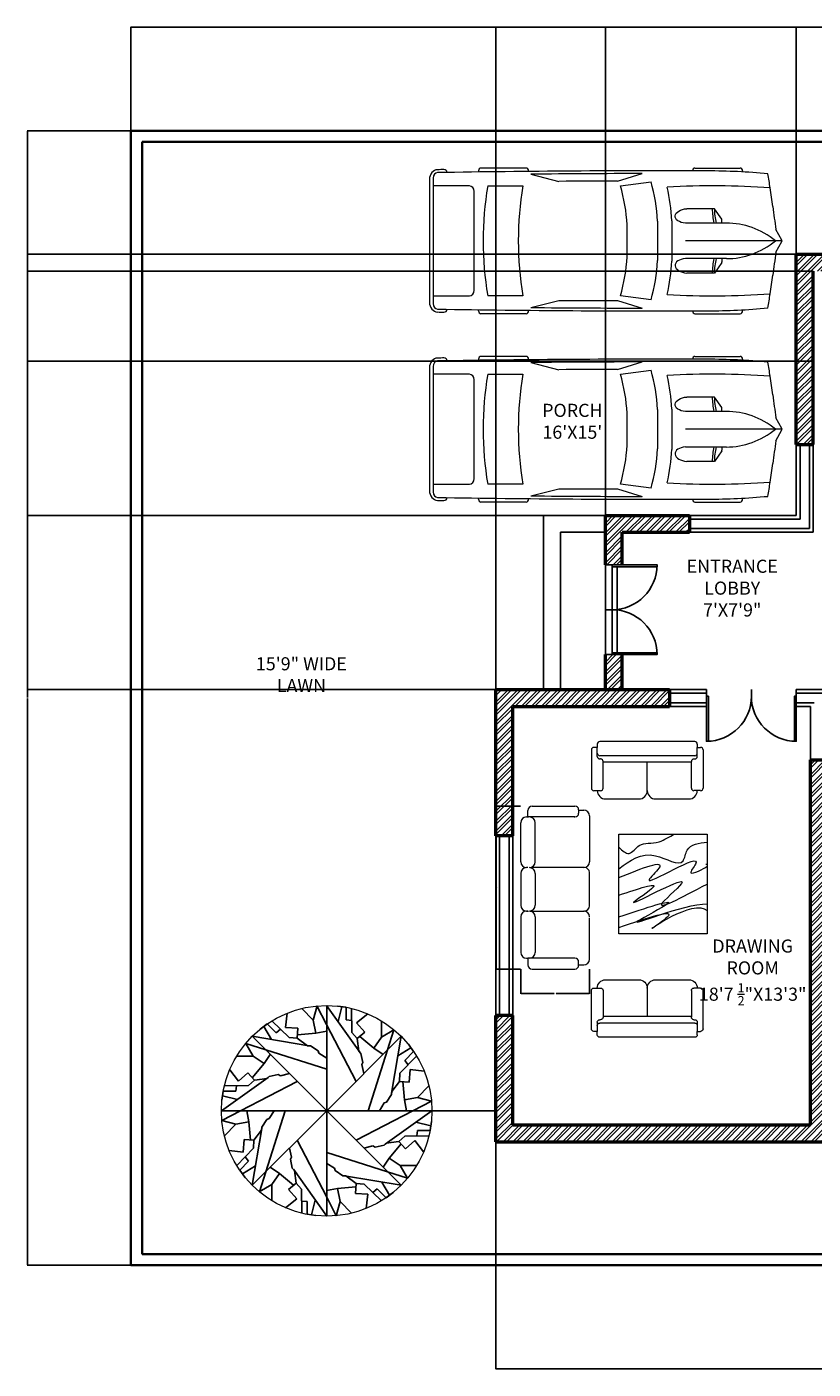
# Model space of a CAD drawing. Units: inches. Extents: x -249 to 953, y -127 to 590.
# Tile 1 of 4: x -249 to 171, y -127 to 590. Entities that reach past the tile are written whole.
import ezdxf

# ---------------------------------------------------------------- set-up
doc = ezdxf.new("R2010")
doc.units = ezdxf.units.IN
doc.header["$MEASUREMENT"] = 0
for name, color, linetype, lineweight in [('A-ANNO-DIMS', 2, 'Continuous', 18), ('A-AREA-IDEN', 2, 'Continuous', 18), ('A-EQPM-VEHC', 8, 'Continuous', 13), ('A-FLOR-STRS', 4, 'Continuous', 25), ('A-FURN', 42, 'Continuous', 18), ('A-GLAZ', 5, 'Continuous', 25), ('A-WALL', 7, 'Continuous', 50), ('A-WALL-PATT', 8, 'Continuous', 13), ('C-PROP', 7, 'Continuous', 35), ('DOOR', 22, 'Continuous', 25), ('L-ANNO-TEXT', 2, 'Continuous', 18), ('L-PLNT', 109, 'Continuous', 18)]:
    doc.layers.add(name, color=color, linetype=linetype, lineweight=lineweight)
doc.layers.add('GREE', color=109, linetype='Continuous')
doc.styles.get("Standard").update_dxf_attribs({"font": 'arial.ttf'})
doc.dimstyles.get("Standard").update_dxf_attribs({"dimtxt": 0.18, "dimasz": 0.18, "dimexe": 0.18, "dimexo": 0.0625, "dimgap": 0.09, "dimtad": 0, "dimtih": 1, "dimtoh": 1, "dimdec": 4, "dimzin": 0, "dimdsep": 46, "dimtxsty": 'Standard', "dimcen": 0.09, "dimadec": 0, "dimazin": 0, "dimtfac": 1, "dimtdec": 4, "dimtofl": 0, "dimtmove": 0, "dimatfit": 3, "dimfxl": 1, "dimtolj": 1, "dimtzin": 0, "dimarcsym": 0})

# ---------------------------------------------------------------- blocks, each defined once
blk = doc.blocks.new('*U2')
for p, q in [((0, 0), (0, -6)), ((40, 0), (40, -6))]:
    blk.add_line(p, q)
blk.add_lwpolyline([(0, 0), (0, 40), (1.75, 40), (1.75, 0)], close=True)
blk.add_arc((0, 0), 40, 0, 90)
blk = doc.blocks.new('A$C0876780F')
for p, q in [((0.72, 0.95), (0.23, 0.95)), ((1.32, 0.95), (0.88, 0.95)), ((1.48, 0.95), (2.02, 0.95)), ((0, 0.79), (0, 0.21)), ((0.15, 0.85), (0.06, 0.85)), ((0.15, 0.87), (0.15, 0.844)), ((0.15, 0.87), (0.15, 0.85)), ((0.15, 0.21), (0.15, 0.85)), ((0.72, 0.75), (0.23, 0.75)), ((0.8, 0.85), (0.8, 0.87)), ((0.8, 0.87), (0.8, 0.85)), ((0.8, 0.87), (0.8, 0.844)), ((0.801, 0.82), (0.801, 0.08)), ((1.32, 0.75), (0.88, 0.75)), ((1.4, 0.85), (1.4, 0.87)), ((1.4, 0.85), (1.4, 0.87)), ((1.401, 0.08), (1.401, 0.803)), ((1.48, 0.75), (2.02, 0.75)), ((2.1, 0.87), (2.1, 0.85)), ((2.1, 0.87), (2.1, 0.844)), ((2.1, 0.21), (2.1, 0.85)), ((2.1, 0.85), (2.19, 0.85)), ((2.25, 0.79), (2.25, 0.21)), ((0, 0.21), (0, 0.2)), ((0.15, 0.2), (0.15, 0.25)), ((2.1, 0.2), (2.1, 0.25)), ((2.25, 0.21), (2.25, 0.2)), ((0.05, 0.15), (0.1, 0.15)), ((0.056, 0.15), (0.056, 0.08)), ((0.136, 0), (0.709, 0)), ((0.801, 0.07), (0.801, 0.08)), ((0.871, 0), (1.331, 0)), ((1.401, 0.07), (1.401, 0.08)), ((2.114, 0), (1.48, 0)), ((2.2, 0.15), (2.15, 0.15)), ((2.194, 0.15), (2.194, 0.08))]:
    blk.add_line(p, q)
for centre, radius, start, end in [((0.23, 0.87), 0.08, 90, 180), ((0.72, 0.87), 0.08, 0, 90), ((0.88, 0.87), 0.08, 90, 180), ((1.32, 0.87), 0.08, 0, 90), ((1.48, 0.87), 0.08, 90, 180), ((2.02, 0.87), 0.08, 0, 90), ((0.06, 0.79), 0.06, 90, 180), ((0.23, 0.83), 0.08, 180, 270), ((0.23, 0.83), 0.08, 180, 270), ((0.72, 0.83), 0.08, 270, 0), ((0.88, 0.83), 0.08, 180, 270), ((0.88, 0.83), 0.08, 180, 270), ((1.32, 0.83), 0.08, 270, 0), ((1.48, 0.83), 0.08, 180, 270), ((2.02, 0.83), 0.08, 270, 0), ((2.02, 0.83), 0.08, 270, 0), ((2.19, 0.79), 0.06, 0, 90), ((0.05, 0.2), 0.05, 180, 270), ((0.1, 0.2), 0.05, 270, 0), ((0.09, 0.21), 0.06, 350.5377, 0), ((2.16, 0.21), 0.06, 180, 189.4623), ((2.15, 0.2), 0.05, 180, 270), ((2.2, 0.2), 0.05, 270, 0), ((0.136, 0.08), 0.08, 180, 270), ((0.721, 0.08), 0.08, 270, 0), ((0.871, 0.07), 0.07, 180, 270), ((1.331, 0.07), 0.07, 270, 0), ((1.481, 0.08), 0.08, 180, 270), ((2.114, 0.08), 0.08, 270, 0)]:
    blk.add_arc(centre, radius, start, end)
blk = doc.blocks.new('A$C02A636C4')
for p, q in [((0.068, 0.64), (0.068, 0.601)), ((1.203, 0.669), (0.097, 0.669)), ((1.232, 0.64), (1.232, 0.601)), ((0, 0.572), (0, 0.126)), ((0.068, 0.601), (0.029, 0.601)), ((0.068, 0.533), (0.068, 0.601)), ((0.068, 0.495), (0.068, 0.543)), ((1.203, 0.504), (0.097, 0.504)), ((1.232, 0.601), (1.271, 0.601)), ((1.232, 0.533), (1.232, 0.601)), ((1.232, 0.495), (1.232, 0.543)), ((1.3, 0.572), (1.3, 0.126)), ((0.107, 0.466), (0.097, 0.466)), ((0.136, 0.126), (0.136, 0.436)), ((1.164, 0.427), (0.136, 0.427)), ((0.65, 0.097), (0.65, 0.427)), ((1.164, 0.126), (1.164, 0.436)), ((1.193, 0.466), (1.203, 0.466)), ((0.029, 0.097), (0.107, 0.097)), ((0.165, 0), (0.553, 0)), ((0.747, 0), (1.135, 0)), ((1.271, 0.097), (1.193, 0.097))]:
    blk.add_line(p, q)
for centre, radius, start, end in [((0.097, 0.64), 0.0291, 90, 180), ((1.203, 0.64), 0.0291, 0, 90), ((0.029, 0.572), 0.0291, 90, 180), ((0.097, 0.533), 0.0291, 180, 270), ((0.097, 0.495), 0.0291, 180, 270), ((1.203, 0.533), 0.0291, 270, 0), ((1.203, 0.495), 0.0291, 270, 0), ((1.271, 0.572), 0.0291, 0, 90), ((0.107, 0.436), 0.0291, 0, 90), ((1.193, 0.436), 0.0291, 90, 180), ((0.029, 0.126), 0.0291, 180, 270), ((0.165, 0.097), 0.097, 180, 270), ((0.107, 0.126), 0.0291, 270, 0), ((0.553, 0.097), 0.097, 270, 0), ((0.747, 0.097), 0.097, 180, 270), ((1.135, 0.097), 0.097, 270, 0), ((1.193, 0.126), 0.0291, 180, 270), ((1.271, 0.126), 0.0291, 270, 0)]:
    blk.add_arc(centre, radius, start, end)
blk = doc.blocks.new('*U13')
for p, q in [((21.1, 37.41), (21.1, 36.83)), ((46.55, 38.89), (22.35, 38.89)), ((47.8, 37.39), (47.8, 37.41)), ((87.99, 31.87), (74.76, 35.92)), ((135.45, 37.07), (135.45, 37.41)), ((136.7, 38.89), (160.9, 38.89)), ((162.15, 37.41), (162.15, 36.77)), ((70.03, 31.54), (86.41, 29.35)), ((134.31, 35.6), (119.29, 31.78)), ((138.42, 29.35), (157.25, 29.35)), ((186.47, 29.35), (167.01, 29.35)), ((186.47, -33.5), (186.47, 33.5)), ((188.4, -32.76), (188.4, 32.76)), ((164.52, 26.39), (164.52, -26.39)), ((32.27, 11.63), (36.13, 17.17)), ((36.13, 17.17), (50.94, 17.17)), ((29.77, 9.51), (51.68, 9.51)), ((32.12, 9.51), (32.12, 11.15)), ((58.92, -10.77), (58.92, 10.77)), ((66.55, -10.53), (66.55, 10.53)), ((82.74, 8.5), (82.74, -8.5)), ((186.47, -10.53), (186.47, 10.53)), ((3.27, 6.13), (0.1, 0.41)), ((0, 0), (51.68, 0)), ((0.1, -0.41), (3.27, -6.13)), ((29.77, -9.51), (51.68, -9.51)), ((32.12, -9.51), (32.12, -11.15)), ((32.27, -11.63), (36.13, -17.17)), ((36.13, -17.17), (50.94, -17.17)), ((86.41, -29.35), (70.03, -31.54)), ((87.99, -31.87), (74.76, -35.92)), ((134.31, -35.6), (119.29, -31.78)), ((157.25, -29.35), (138.42, -29.35)), ((167.01, -29.35), (186.47, -29.35)), ((21.1, -37.41), (21.1, -36.83)), ((46.55, -38.89), (22.35, -38.89)), ((47.8, -37.39), (47.8, -37.41)), ((135.45, -37.07), (135.45, -37.41)), ((136.7, -38.89), (160.9, -38.89)), ((162.15, -37.41), (162.15, -36.77))]:
    blk.add_line(p, q)
for centre, major_axis, ratio, start_param, end_param in [((266.03, -27.52), (0, 313.31), 0.842304, 1.367076, 1.39176), ((41.19, -490.86), (0, 528.23), 0.842304, 0.00281, 0.075598), ((22.35, 37.41), (0, -1.48), 0.842304, 3.141593, 4.712389), ((64.48, -10555.62), (0, 10593.03), 0.842304, -0.013397, 0.002797), ((46.55, 37.41), (0, 1.48), 0.842304, -1.570796, 0), ((64.48, -10555.62), (0, -10591.55), 0.842304, 3.133765, 3.140441), ((136.7, 37.41), (0, -1.48), 0.842304, 3.141593, 4.712389), ((160.9, 37.41), (0, 1.48), 0.842304, -1.570796, 0), ((180.63, 35.84), (0, 2.22), 0.842304, -0.013017, 1.249894), ((64.48, -10556.36), (0, 10595.31), 0.842304, -0.013397, -0.013017), ((183.98, 33.5), (0, -2.96), 0.842304, 1.570796, 3.128196), ((183.98, 32.76), (0, -5.25), 0.842304, 1.570796, 3.128196), ((37.47, -593.96), (0, -623.33), 0.842304, 3.096046, 3.200911), ((134.4, 5.39), (0, -89.78), 0.842304, 4.449482, 4.652344), ((135.29, 5.39), (0, 81.77), 0.842304, 1.245306, 1.50788), ((149.6, 2.8), (0, -79.58), 0.842304, 4.372215, 4.640744), ((95.79, -3666.35), (0, -3698.24), 0.842304, 3.134049, 3.144098), ((17.08, 0), (0, 147.02), 0.842304, 4.511394, 4.913384), ((35.91, 0), (0, 147.02), 0.842304, 4.511394, 4.913384), ((167.01, 26.39), (0, 2.96), 0.842304, 0, 1.570796), ((259.18, -27.52), (0, -305.3), 0.842304, 4.528606, 4.561838), ((-204.49, 52.4), (0, -250.96), 0.842304, 1.385369, 1.434372), ((13.04, 17.01), (0, 27.42), 0.842304, 4.435146, 4.718221), ((14.2, 17.01), (0, 27.42), 0.842304, 4.435146, 4.718221), ((50.79, 13.34), (6.34, -0.36), 0.603834, -1.395552, 1.581315), ((29.77, -46.66), (0, 56.17), 0.842304, 0, 0.590319), ((32.75, 11.15), (0, 0.74), 0.842304, 0.879714, 1.570796), ((0.62, 0), (0, -0.74), 0.842304, 4.131459, 5.293319), ((-204.49, -52.4), (0, 250.96), 0.842304, -1.434372, -1.385369), ((29.77, 46.66), (0, 56.17), 0.842304, 2.551274, 3.141593), ((32.75, -11.15), (0, -0.74), 0.842304, 4.712389, 5.403472), ((13.04, -17.01), (0, -27.42), 0.842304, 1.564964, 1.848039), ((14.2, -17.01), (0, -27.42), 0.842304, 1.564964, 1.848039), ((134.4, -5.39), (0, -89.78), 0.842304, -1.510751, -1.307889), ((135.29, -5.39), (0, -81.77), 0.842304, -1.50788, -1.245306), ((149.6, -2.8), (0, -79.58), 0.842304, -1.499151, -1.230623), ((259.18, 27.52), (0, 305.3), 0.842304, 1.721348, 1.754579), ((266.03, 27.52), (0, 313.31), 0.842304, 1.749832, 1.774517), ((37.47, 593.96), (0, -623.33), 0.842304, -0.059319, 0.045547), ((167.01, -26.39), (0, -2.96), 0.842304, 4.712389, 6.283185), ((64.48, 10555.62), (0, -10591.55), 0.842304, 0.001152, 0.007828), ((95.79, 3666.35), (0, -3698.24), 0.842304, -0.002505, 0.007544), ((183.98, -33.5), (0, 2.96), 0.842304, 3.15499, 4.712389), ((183.98, -32.76), (0, -5.25), 0.842304, 0.013397, 1.570796), ((41.19, 490.86), (0, -528.23), 0.842304, -0.075598, -0.00281), ((22.35, -37.41), (0, 1.48), 0.842304, 1.570796, 3.141593), ((64.48, 10555.62), (0, 10593.03), 0.842304, 3.138796, 3.15499), ((46.55, -37.41), (0, -1.48), 0.842304, 0, 1.570796), ((136.7, -37.41), (0, -1.48), 0.842304, -1.570796, 0), ((160.9, -37.41), (0, 1.48), 0.842304, 3.141593, 4.712389), ((180.63, -35.84), (0, -2.22), 0.842304, -1.249894, 0.013017), ((64.48, 10556.36), (0, 10595.31), 0.842304, 3.15461, 3.15499)]:
    blk.add_ellipse(centre, major_axis=major_axis, ratio=ratio, start_param=start_param, end_param=end_param)
at = {"extrusion": (0, 0, -1)}
blk.add_ellipse((50.79, -13.34), major_axis=(6.34, 0.36), ratio=0.603834, start_param=-1.395552, end_param=1.581315, dxfattribs=at)
blk = doc.blocks.new('*U21')
at = {"layer": 'GREE'}
blk.add_line((28.13, 0), (-28.13, 0), dxfattribs=at)
blk = doc.blocks.new('*U22')
at = {"layer": 'L-PLNT', "transparency": 16777216}
for p, rotation in [((-88.7, 39.57), 90), ((-108.59, 31.33), 135), ((-68.81, 31.33), 45), ((-116.83, 11.44), 180), ((-108.59, -8.46), 225), ((-88.7, -16.7), 270), ((-68.81, -8.46), 315)]:
    blk.add_blockref('*U21', p, dxfattribs=dict(at, rotation=rotation))
blk.add_blockref('*U21', (-60.57, 11.44), dxfattribs=at)
blk = doc.blocks.new('*U23')
at = {"layer": 'GREE'}
for p, q in [((-15.41, 10.07), (-20.57, 20.04)), ((2.4, -4.73), (-15.41, 20.28)), ((-4.98, 19.3), (-9.66, 19.98)), ((-9.32, 11.73), (-7.32, 19.64)), ((-4.98, 12.53), (-4.98, 19.3)), ((-1.91, 5.84), (-2.1, 18.68)), ((0.51, 11.09), (6.52, 15.83)), ((0.3, -20.28), (-15.41, 10.07)), ((-2, 12.26), (-4.98, 12.53)), ((4.9, 6.07), (0.51, 11.09)), ((13.81, 3.32), (13.81, 12.1)), ((13.81, 3.32), (20.57, 7.27)), ((0.93, 2.6), (-1.91, 5.84)), ((0.93, 2.6), (4.9, 6.07)), ((1.86, -4.12), (0.93, 2.6)), ((9.84, -2.53), (2.27, 3.77)), ((9.84, -2.53), (13.81, 3.32)), ((2.94, -5.33), (1.86, -4.12)), ((3.93, -10.13), (2.94, -5.33)), ((14.73, -5.86), (9.84, -2.53)), ((3.36, -11.31), (3.93, -10.13)), ((4.49, -16.09), (3.36, -11.31))]:
    blk.add_line(p, q, dxfattribs=at)
blk = doc.blocks.new('*U24')
at = {"layer": 'L-PLNT', "transparency": 16777216}
for p, rotation in [((-103.25, 47.78), 45.00000000000002), ((-52.36, 25.99), 315), ((-124.69, 26.84), 90.00000000000006), ((-125.04, -3.12), 135), ((-52.71, -3.97), 270), ((-74.15, -24.9), 225), ((-104.11, -24.55), 180)]:
    blk.add_blockref('*U23', p, dxfattribs=dict(at, rotation=rotation))
blk.add_blockref('*U23', (-73.3, 47.42), dxfattribs=at)
blk = doc.blocks.new('TABLE-COFFEE-PATTERNED')
blk.add_lwpolyline([(0, 53.34), (47.12, 53.34), (47.12, 0), (0, 0)], close=True)
for points, knots in [([(0, 46.27), (1.84, 44.53), (5.7, 40.88), (11.7, 50.21), (19.06, 46.91), (27.14, 52), (29.62, 53.34)], [0, 0, 0, 0, 6.282368, 13.190835, 24.063381, 30.451568, 30.451568, 30.451568, 30.451568]), ([(0, 34.85), (5.86, 39.26), (15.94, 46.83), (34.57, 34.01), (35.96, 47.88), (42.72, 48.56), (47.12, 49)], [0, 0, 0, 0, 20.758426, 35.677626, 41.810907, 53.27251, 53.27251, 53.27251, 53.27251]), ([(0, 30.13), (12.39, 35.14), (29.39, 42), (5.27, 19.44), (51.08, 48.6), (34.79, 29.62), (45.43, 34.67), (47.12, 36.21)], [0, 0, 0, 0, 21.871026, 29.981696, 56.235396, 61.567804, 69.030503, 69.030503, 69.030503, 69.030503]), ([(0, 20.7), (10.31, 24.19), (27.82, 30.11), (-7.6, 7.42), (48.95, 38.75), (11.44, 7.85), (33.32, 19.39), (47.12, 26.67)], [0, 0, 0, 0, 18.796744, 31.916986, 59.888518, 75.000199, 100.823224, 100.823224, 100.823224, 100.823224]), ([(0, 3.52), (15.31, 8.65), (36.14, 15.62), (5.39, -5.65), (40.11, 19.54), (47.12, 12.46)], [0, 0, 0, 0, 26.265752, 35.743864, 66.169502, 66.169502, 66.169502, 66.169502]), ([(0, 9.16), (14.7, 14.03), (39.32, 22.19), (-9.44, -2.68), (34.4, 16.08), (47.12, 16.13)], [0, 0, 0, 0, 26.807232, 44.891452, 82.87087, 82.87087, 82.87087, 82.87087])]:
    blk.add_open_spline(points, degree=3, knots=knots)
blk.add_open_spline([(47.12, 37.08), (46.93, 37.1), (46.67, 37.09), (46.41, 37.08)], degree=3)
blk = doc.blocks.new('WIN-96IN')
for p, q in [((0, 9), (96, 9)), ((0, 7), (96, 7)), ((0, 2), (96, 2)), ((0, 0), (96, 0))]:
    blk.add_line(p, q)
blk = doc.blocks.new('*D31')
at = {"layer": 'A-ANNO-DIMS', "color": 0, "lineweight": -2, "transparency": 16777216}
for p, q in [((14.9, 174.21), (1.72, 174.21)), ((1.9, 174.03), (1.9, 130.87)), ((1.9, 87.35), (1.9, 130.5)), ((14.9, 87.17), (1.72, 87.17))]:
    blk.add_line(p, q, dxfattribs=at)
at = {"layer": 'A-ANNO-DIMS', "color": 0, "transparency": 16777216}
for points in [[(1.87, 174.03), (1.93, 174.03), (1.9, 174.21)], [(1.87, 87.35), (1.93, 87.35), (1.9, 87.17)]]:
    blk.add_solid(points, dxfattribs=at)
at = {"layer": 'Defpoints', "color": 0, "transparency": 16777216}
for p in [(1.9, 174.21), (14.96, 174.21), (14.96, 87.17)]:
    blk.add_point(p, dxfattribs=at)
at = {"layer": 'A-ANNO-DIMS', "color": 0, "transparency": 16777216, "insert": (1.9, 130.69), "char_height": 0.18, "attachment_point": 5}
blk.add_mtext('\\A1;SOFA 87 TYP.', dxfattribs=at)
blk = doc.blocks.new('*D32')
at = {"layer": 'A-ANNO-DIMS', "color": 0, "lineweight": -2, "transparency": 16777216}
for p, q in [((14.96, 87.11), (14.96, 73.93)), ((51.71, 87.11), (51.71, 73.93)), ((15.14, 74.11), (32.81, 74.11)), ((51.53, 74.11), (33.86, 74.11))]:
    blk.add_line(p, q, dxfattribs=at)
at = {"layer": 'A-ANNO-DIMS', "color": 0, "transparency": 16777216}
for points in [[(15.14, 74.14), (15.14, 74.08), (14.96, 74.11)], [(51.53, 74.14), (51.53, 74.08), (51.71, 74.11)]]:
    blk.add_solid(points, dxfattribs=at)
at = {"layer": 'Defpoints', "color": 0, "transparency": 16777216}
for p in [(14.96, 87.17), (51.71, 87.17), (14.96, 74.11)]:
    blk.add_point(p, dxfattribs=at)
at = {"layer": 'A-ANNO-DIMS', "color": 0, "transparency": 16777216, "insert": (33.34, 74.11), "char_height": 0.18, "attachment_point": 5}
blk.add_mtext('\\A1;37 TYP.', dxfattribs=at)
blk = doc.blocks.new('*D51')
at = {"layer": 'A-ANNO-DIMS', "color": 0, "lineweight": -2, "transparency": 16777216}
for p, q in [((-193.28, 534.99), (-193.28, 590.41)), ((-193.1, 590.23), (351.51, 590.23)), ((897.04, 590.23), (352.42, 590.23)), ((897.22, 534.99), (897.22, 590.41))]:
    blk.add_line(p, q, dxfattribs=at)
at = {"layer": 'A-ANNO-DIMS', "color": 0, "transparency": 16777216}
for points in [[(-193.1, 590.26), (-193.1, 590.2), (-193.28, 590.23)], [(897.04, 590.26), (897.04, 590.2), (897.22, 590.23)]]:
    blk.add_solid(points, dxfattribs=at)
at = {"layer": 'Defpoints', "color": 0, "transparency": 16777216}
for p in [(897.22, 590.23), (-193.28, 534.93), (897.22, 534.93)]:
    blk.add_point(p, dxfattribs=at)
at = {"layer": 'A-ANNO-DIMS', "color": 0, "transparency": 16777216, "insert": (351.97, 590.23), "char_height": 0.18, "attachment_point": 5}
blk.add_mtext('\\A1;1090.5', dxfattribs=at)
blk = doc.blocks.new('*D52')
at = {"layer": 'A-ANNO-DIMS', "color": 0, "lineweight": -2, "transparency": 16777216}
for p, q in [((-193.35, 534.93), (-248.76, 534.93)), ((-248.58, 534.75), (-248.58, 232.11)), ((-248.58, -70.89), (-248.58, 231.75)), ((-193.35, -71.07), (-248.76, -71.07))]:
    blk.add_line(p, q, dxfattribs=at)
at = {"layer": 'A-ANNO-DIMS', "color": 0, "transparency": 16777216}
for points in [[(-248.61, 534.75), (-248.55, 534.75), (-248.58, 534.93)], [(-248.61, -70.89), (-248.55, -70.89), (-248.58, -71.07)]]:
    blk.add_solid(points, dxfattribs=at)
at = {"layer": 'Defpoints', "color": 0, "transparency": 16777216}
for p in [(-248.58, 534.93), (-193.28, 534.93), (-193.28, -71.07)]:
    blk.add_point(p, dxfattribs=at)
at = {"layer": 'A-ANNO-DIMS', "color": 0, "transparency": 16777216, "insert": (-248.58, 231.93), "char_height": 0.18, "attachment_point": 5}
blk.add_mtext('\\A1;606', dxfattribs=at)
blk = doc.blocks.new('*D53')
at = {"layer": 'A-ANNO-DIMS', "color": 0, "lineweight": -2, "transparency": 16777216}
for p, q in [((1.72, -5.13), (1.72, -126.55)), ((831.22, -5.13), (831.22, -126.55)), ((1.9, -126.37), (416.07, -126.37)), ((831.04, -126.37), (416.86, -126.37))]:
    blk.add_line(p, q, dxfattribs=at)
at = {"layer": 'A-ANNO-DIMS', "color": 0, "transparency": 16777216}
for points in [[(1.9, -126.34), (1.9, -126.4), (1.72, -126.37)], [(831.04, -126.34), (831.04, -126.4), (831.22, -126.37)]]:
    blk.add_solid(points, dxfattribs=at)
at = {"layer": 'Defpoints', "color": 0, "transparency": 16777216}
for p in [(1.72, -5.07), (831.22, -5.07), (831.22, -126.37)]:
    blk.add_point(p, dxfattribs=at)
at = {"layer": 'A-ANNO-DIMS', "color": 0, "transparency": 16777216, "insert": (416.47, -126.37), "char_height": 0.18, "attachment_point": 5}
blk.add_mtext('\\A1;829.5', dxfattribs=at)
blk = doc.blocks.new('*D55')
at = {"layer": 'A-ANNO-DIMS', "color": 0, "lineweight": -2, "transparency": 16777216}
for p, q in [((1.72, 236.49), (1.72, 590.41)), ((1.9, 590.23), (30.64, 590.23)), ((60.04, 590.23), (31.29, 590.23)), ((60.22, 236.49), (60.22, 590.41))]:
    blk.add_line(p, q, dxfattribs=at)
at = {"layer": 'A-ANNO-DIMS', "color": 0, "transparency": 16777216}
for points in [[(1.9, 590.26), (1.9, 590.2), (1.72, 590.23)], [(60.04, 590.26), (60.04, 590.2), (60.22, 590.23)]]:
    blk.add_solid(points, dxfattribs=at)
at = {"layer": 'Defpoints', "color": 0, "transparency": 16777216}
for p in [(60.22, 590.23), (1.72, 236.43), (60.22, 236.43)]:
    blk.add_point(p, dxfattribs=at)
at = {"layer": 'A-ANNO-DIMS', "color": 0, "transparency": 16777216, "insert": (30.97, 590.23), "char_height": 0.18, "attachment_point": 5}
blk.add_mtext('\\A1;58.5', dxfattribs=at)
blk = doc.blocks.new('*D56')
at = {"layer": 'A-ANNO-DIMS', "color": 0, "lineweight": -2, "transparency": 16777216}
for p, q in [((60.22, 329.49), (60.22, 590.41)), ((60.4, 590.23), (110.94, 590.23)), ((162.04, 590.23), (111.5, 590.23)), ((162.22, 329.49), (162.22, 590.41))]:
    blk.add_line(p, q, dxfattribs=at)
at = {"layer": 'A-ANNO-DIMS', "color": 0, "transparency": 16777216}
for points in [[(60.4, 590.26), (60.4, 590.2), (60.22, 590.23)], [(162.04, 590.26), (162.04, 590.2), (162.22, 590.23)]]:
    blk.add_solid(points, dxfattribs=at)
at = {"layer": 'Defpoints', "color": 0, "transparency": 16777216}
for p in [(162.22, 590.23), (60.22, 329.43), (162.22, 329.43)]:
    blk.add_point(p, dxfattribs=at)
at = {"layer": 'A-ANNO-DIMS', "color": 0, "transparency": 16777216, "insert": (111.22, 590.23), "char_height": 0.18, "attachment_point": 5}
blk.add_mtext('\\A1;102', dxfattribs=at)
blk = doc.blocks.new('*D57')
at = {"layer": 'A-ANNO-DIMS', "color": 0, "lineweight": -2, "transparency": 16777216}
for p, q in [((60.15, 329.43), (-248.76, 329.43)), ((-248.58, 329.25), (-248.58, 283.11)), ((-248.58, 236.61), (-248.58, 282.75)), ((60.15, 236.43), (-248.76, 236.43))]:
    blk.add_line(p, q, dxfattribs=at)
at = {"layer": 'A-ANNO-DIMS', "color": 0, "transparency": 16777216}
for points in [[(-248.61, 329.25), (-248.55, 329.25), (-248.58, 329.43)], [(-248.61, 236.61), (-248.55, 236.61), (-248.58, 236.43)]]:
    blk.add_solid(points, dxfattribs=at)
at = {"layer": 'Defpoints', "color": 0, "transparency": 16777216}
for p in [(-248.58, 329.43), (60.22, 329.43), (60.22, 236.43)]:
    blk.add_point(p, dxfattribs=at)
at = {"layer": 'A-ANNO-DIMS', "color": 0, "transparency": 16777216, "insert": (-248.58, 282.93), "char_height": 0.18, "attachment_point": 5}
blk.add_mtext('\\A1;93', dxfattribs=at)
blk = doc.blocks.new('*D58')
at = {"layer": 'A-ANNO-DIMS', "color": 0, "lineweight": -2, "transparency": 16777216}
for p, q in [((162.15, 468.93), (-248.76, 468.93)), ((-248.58, 468.75), (-248.58, 399.36)), ((-248.58, 329.61), (-248.58, 399)), ((162.15, 329.43), (-248.76, 329.43))]:
    blk.add_line(p, q, dxfattribs=at)
at = {"layer": 'A-ANNO-DIMS', "color": 0, "transparency": 16777216}
for points in [[(-248.61, 468.75), (-248.55, 468.75), (-248.58, 468.93)], [(-248.61, 329.61), (-248.55, 329.61), (-248.58, 329.43)]]:
    blk.add_solid(points, dxfattribs=at)
at = {"layer": 'Defpoints', "color": 0, "transparency": 16777216}
for p in [(-248.58, 468.93), (162.22, 468.93), (162.22, 329.43)]:
    blk.add_point(p, dxfattribs=at)
at = {"layer": 'A-ANNO-DIMS', "color": 0, "transparency": 16777216, "insert": (-248.58, 399.18), "char_height": 0.18, "attachment_point": 5}
blk.add_mtext('\\A1;139.5', dxfattribs=at)
blk = doc.blocks.new('*D61')
at = {"layer": 'A-ANNO-DIMS', "color": 0, "lineweight": -2, "transparency": 16777216}
for p, q in [((171.15, 459.93), (-248.76, 459.93)), ((-248.58, 459.75), (-248.58, 436.11)), ((-248.58, 412.11), (-248.58, 435.75)), ((171.15, 411.93), (-248.76, 411.93))]:
    blk.add_line(p, q, dxfattribs=at)
at = {"layer": 'A-ANNO-DIMS', "color": 0, "transparency": 16777216}
for points in [[(-248.61, 459.75), (-248.55, 459.75), (-248.58, 459.93)], [(-248.61, 412.11), (-248.55, 412.11), (-248.58, 411.93)]]:
    blk.add_solid(points, dxfattribs=at)
at = {"layer": 'Defpoints', "color": 0, "transparency": 16777216}
for p in [(-248.58, 459.93), (171.22, 459.93), (171.22, 411.93)]:
    blk.add_point(p, dxfattribs=at)
at = {"layer": 'A-ANNO-DIMS', "color": 0, "transparency": 16777216, "insert": (-248.58, 435.93), "char_height": 0.18, "attachment_point": 5}
blk.add_mtext('\\A1;48', dxfattribs=at)
blk = doc.blocks.new('*D62')
at = {"layer": 'A-ANNO-DIMS', "color": 0, "lineweight": -2, "transparency": 16777216}
for p, q in [((162.22, 468.99), (162.22, 590.41)), ((162.4, 590.23), (171.78, 590.23)), ((182.09, 590.23), (172.71, 590.23)), ((182.27, 468.99), (182.27, 590.41))]:
    blk.add_line(p, q, dxfattribs=at)
at = {"layer": 'A-ANNO-DIMS', "color": 0, "transparency": 16777216}
for points in [[(162.4, 590.26), (162.4, 590.2), (162.22, 590.23)], [(182.09, 590.26), (182.09, 590.2), (182.27, 590.23)]]:
    blk.add_solid(points, dxfattribs=at)
at = {"layer": 'Defpoints', "color": 0, "transparency": 16777216}
for p in [(182.27, 590.23), (162.22, 468.93), (182.27, 468.93)]:
    blk.add_point(p, dxfattribs=at)
at = {"layer": 'A-ANNO-DIMS', "color": 0, "transparency": 16777216, "insert": (172.24, 590.23), "char_height": 0.18, "attachment_point": 5}
blk.add_mtext('\\A1;20.058', dxfattribs=at)
blk = doc.blocks.new('*D67')
at = {"layer": 'A-ANNO-DIMS', "color": 0, "lineweight": -2, "transparency": 16777216}
for p, q in [((-88.79, 11.44), (-88.61, 11.44)), ((-88.7, 11.35), (-88.7, 11.53)), ((1.32, 11.44), (-32.26, 11.44))]:
    blk.add_line(p, q, dxfattribs=at)
at = {"layer": 'A-ANNO-DIMS', "color": 0, "transparency": 16777216}
blk.add_solid([(-32.26, 11.47), (-32.26, 11.41), (-32.44, 11.44)], dxfattribs=at)
at = {"layer": 'Defpoints', "color": 0, "transparency": 16777216}
for p in [(-144.97, 11.44), (-32.44, 11.44)]:
    blk.add_point(p, dxfattribs=at)
at = {"layer": 'A-ANNO-DIMS', "color": 0, "transparency": 16777216, "insert": (1.88, 11.44), "char_height": 0.18, "attachment_point": 5}
blk.add_mtext('\\A1;∅112.53', dxfattribs=at)

msp = doc.modelspace()

# ---------------------------------------------------------------- hatches: boundary and pattern name
at = {"layer": 'A-WALL-PATT'}
h = msp.add_hatch(dxfattribs=at)
h.set_pattern_fill('ANSI32', color=256, scale=10)
h.paths.add_polyline_path([(387.3054, 468.9306), (318.2157, 468.9306), (318.2157, 459.9306), (387.3054, 459.9306)])
h.paths.add_polyline_path([(327.2157, 459.9306), (318.2157, 459.9306), (318.2157, 262.174), (321.8157, 262.174), (327.2157, 262.174)])
h.paths.add_polyline_path([(318.2157, 468.9306), (212.2733, 468.9306), (212.2733, 459.9306), (318.2157, 459.9306)])
h.paths.add_polyline_path([(182.2733, 468.9306), (162.2157, 468.9306), (162.2157, 367.3439), (171.2157, 367.3439), (171.2157, 459.9306), (182.2733, 459.9306)])
h = msp.add_hatch(dxfattribs=at)
h.set_pattern_fill('ANSI32', color=256, scale=10)
h.paths.add_polyline_path([(94.5157, 236.4306), (1.7157, 236.4306), (1.7157, 158.26), (10.7157, 158.26), (10.7157, 227.4306), (94.5157, 227.4306)])
h.paths.add_polyline_path([(69.2157, 255.0908), (63.8157, 255.0908), (60.2157, 255.0908), (60.2157, 236.4306), (69.2157, 236.4306)])
h.paths.add_polyline_path([(105.1039, 329.4306), (60.2157, 329.4306), (60.2157, 303.0908), (63.8157, 303.0908), (69.2157, 303.0908), (69.2157, 320.4306), (105.1039, 320.4306)])
h = msp.add_hatch(dxfattribs=at)
h.set_pattern_fill('ANSI32', color=256, scale=10)
h.paths.add_polyline_path([(442.0897, 207.9306), (417.2157, 207.9306), (417.2157, 198.9306), (442.0897, 198.9306)])
h.paths.add_polyline_path([(411.2157, 207.9306), (340.7157, 207.9306), (340.7157, 198.9306), (411.2157, 198.9306)])
h.paths.add_polyline_path([(340.7157, 207.9306), (334.7157, 207.9306), (334.7157, 180.6902), (338.9157, 180.6902), (340.7157, 180.6902)])
h.paths.add_polyline_path([(334.7157, 198.9306), (295.4153, 198.9306), (295.4153, 189.9306), (334.7157, 189.9306)], flags=17)
h.paths.add_polyline_path([(411.2157, 132.9306), (373.6294, 132.9306), (373.6294, 128.9308, -0.05252224), (373.1027, 123.9306), (411.2157, 123.9306)])
h.paths.add_polyline_path([(340.7157, 152.7481, -0.01608391), (338.9157, 152.6902), (334.7157, 152.6902), (334.7157, 3.9306), (178.7157, 3.9306), (178.7157, 189.9306), (230.1981, 189.9306), (230.1981, 198.9306), (169.7157, 198.9306), (169.7157, 3.9306), (10.7157, 3.9306), (10.7157, 62.26), (1.7157, 62.26), (1.7157, -5.0694), (345.6752, -5.0694), (345.6752, -1.0697), (345.6752, 3.9306), (340.7157, 3.9306)])
h.paths.add_polyline_path([(349.631, 132.9306), (340.7157, 132.9306), (340.7157, 123.9306), (349.631, 123.9306), (349.631, 128.9308)])

# ---------------------------------------------------------------- linework, layer by layer
at = {"layer": 'A-FLOR-STRS'}
for p, q in [((60.2157, 329.4306), (27.2157, 329.4306)), ((27.2157, 329.4306), (27.2157, 236.4306)), ((60.2157, 320.4306), (36.2157, 320.4306)), ((36.2157, 320.4306), (36.2157, 236.4306))]:
    msp.add_line(p, q, dxfattribs=at)
at = {"layer": 'A-GLAZ'}
for p, q in [((162.2157, 367.3439), (162.2157, 329.4306)), ((164.2157, 367.3439), (164.2157, 327.4306)), ((169.2157, 367.3439), (169.2157, 322.4306)), ((171.2157, 367.3439), (171.2157, 320.4306)), ((105.1039, 329.4306), (162.2157, 329.4306)), ((105.1039, 327.4306), (164.2157, 327.4306)), ((105.1039, 322.4306), (169.2157, 322.4306)), ((105.1039, 320.4306), (171.2157, 320.4306)), ((94.5157, 236.4306), (114.2157, 236.4306)), ((94.5157, 234.4306), (114.2157, 234.4306)), ((94.5157, 229.4306), (114.2157, 229.4306)), ((162.2157, 236.4306), (178.7157, 236.4306)), ((162.2157, 234.4306), (176.7157, 234.4306)), ((162.2157, 229.4306), (171.7157, 229.4306)), ((94.5157, 227.4306), (114.2157, 227.4306)), ((162.2157, 227.4306), (169.7157, 227.4306)), ((169.7157, 198.9306), (169.7157, 227.4306))]:
    msp.add_line(p, q, dxfattribs=at)
at = {"layer": 'A-WALL'}
for p, q in [((162.2157, 468.9306), (182.2733, 468.9306)), ((162.2157, 367.3439), (162.2157, 468.9306)), ((171.2157, 367.3439), (171.2157, 459.9306)), ((162.2157, 367.3439), (171.2157, 367.3439)), ((60.2157, 329.4306), (105.1039, 329.4306)), ((60.2157, 303.0908), (60.2157, 329.4306)), ((105.1039, 329.4306), (105.1039, 320.4306)), ((69.2157, 320.4306), (105.1039, 320.4306)), ((69.2157, 303.0908), (69.2157, 320.4306)), ((60.2157, 236.4306), (60.2157, 255.0908)), ((69.2157, 236.4306), (69.2157, 255.0908)), ((1.7157, 236.4306), (94.5157, 236.4306)), ((1.7157, 158.26), (1.7157, 236.4306)), ((94.5157, 236.4306), (94.5157, 227.4306)), ((10.7157, 227.4306), (94.5157, 227.4306)), ((10.7157, 158.26), (10.7157, 227.4306)), ((169.7157, 3.9306), (169.7157, 198.9306)), ((169.7157, 198.9306), (230.1981, 198.9306)), ((10.7157, 158.26), (1.7157, 158.26)), ((1.7157, -5.0694), (1.7157, 62.26)), ((10.7157, 62.26), (1.7157, 62.26)), ((10.7157, 3.9306), (10.7157, 62.26)), ((10.7157, 3.9306), (169.7157, 3.9306)), ((1.7157, -5.0694), (345.6752, -5.0694))]:
    msp.add_line(p, q, dxfattribs=at)
at = {"layer": 'C-PROP'}
for p, q in [((-193.2843, -71.0694), (-193.2843, 534.9306)), ((-193.2843, 534.9306), (897.2157, 534.9306)), ((-187.2843, 528.9306), (891.2157, 528.9306)), ((-187.2843, -65.0694), (-187.2843, 528.9306)), ((-193.2843, -71.0694), (897.2157, -71.0694)), ((-187.2843, -65.0694), (891.2157, -65.0694))]:
    msp.add_line(p, q, dxfattribs=at)
at = {"layer": 'DOOR'}
for p, q in [((63.8157, 302.0408), (63.8157, 256.1408)), ((66.5623, 302.0408), (66.5623, 256.1408))]:
    msp.add_line(p, q, dxfattribs=at)
at = {"layer": 'L-PLNT'}
msp.add_circle((-88.7013, 11.436), 56.2642, dxfattribs=at)

# ---------------------------------------------------------------- block references
at = {"layer": 'A-EQPM-VEHC', "rotation": 180}
for p in [(154.6109, 476.1023), (154.6109, 375.5056)]:
    msp.add_blockref('*U13', p, dxfattribs=at)
at = {"layer": 'A-FURN', "xscale": 45.88752760856259, "yscale": 45.88752760856259, "zscale": 45.88752760856259}
msp.add_blockref('A$C02A636C4', (52.7563, 177.9857), dxfattribs=at)
at = {"layer": 'A-FURN'}
for name, p, xscale, yscale, zscale, rotation in [('A$C0876780F', (51.7095, 87.1689), 38.68315051238548, 38.68315051238548, 38.68315051238548, 90), ('A$C02A636C4', (52.7563, 81.455), -45.88752760856259, 45.88752760856259, 45.88752760856259, 180)]:
    msp.add_blockref(name, p, dxfattribs=dict(at, xscale=xscale, yscale=yscale, zscale=zscale, rotation=rotation))
msp.add_blockref('TABLE-COFFEE-PATTERNED', (67.467, 105.903), dxfattribs=at)
at = {"layer": 'A-GLAZ', "rotation": 90.00000000000003}
msp.add_blockref('WIN-96IN', (10.7153, 62.2596), dxfattribs=at)
at = {"layer": 'DOOR', "yscale": 0.6, "zscale": 0.6}
for p, xscale, rotation in [((63.8157, 303.0908), 0.6, 270), ((63.8157, 255.0908), -0.6, 270), ((114.2157, 232.8306), -0.6, 180), ((162.2157, 232.8306), 0.6, 180)]:
    msp.add_blockref('*U2', p, dxfattribs=dict(at, xscale=xscale, rotation=rotation))
at = {"layer": 'L-PLNT'}
for name in ['*U24', '*U22']:
    msp.add_blockref(name, (0, 0), dxfattribs=at)

# ---------------------------------------------------------------- texts
at = {"layer": 'A-AREA-IDEN', "char_height": 7, "attachment_point": 1}
for s, insert in [("\\A1;\\pxqc;PORCH\\P16'X15'", (2.7501, 389.0712)), ('\\A1;\\pxqc;ENTRANCE\\PLOBBY\\P7\'X7\'9"', (88.1783, 305.7939)), ('\\A1;\\pxqc;DRAWING\\PROOM\\P18\'7 {\\H0.7x;\\S1/2;}"X13\'3"', (99.1058, 102.9449))]:
    msp.add_mtext_dynamic_manual_height_columns(s, width=79.609867, gutter_width=1, heights=[0], dxfattribs=dict(at, insert=insert))
at = {"layer": 'L-ANNO-TEXT', "insert": (-142.0112, 253.716), "char_height": 7, "attachment_point": 1}
msp.add_mtext_dynamic_manual_height_columns('\\A1;\\pxqc;15\'9" WIDE\\PLAWN', width=79.609867, gutter_width=1, heights=[0], dxfattribs=at)

# ---------------------------------------------------------------- dimensions: what is measured, and where the dimension line sits
at = {"layer": 'A-ANNO-DIMS'}
for base, p1, p2, override, picture, middle in [((897.2157, 590.2306), (-193.2843, 534.9306), (897.2157, 534.9306), {"dimdec": 1, "dimlfac": 1, "dimrnd": 0, "dimzin": 0, "dimdsep": 46, "dimlunit": 2}, '*D51', (351.9657, 590.2306)), ((60.2157, 590.2306), (1.7157, 236.4306), (60.2157, 236.4306), {"dimdec": 1, "dimlfac": 1, "dimrnd": 0, "dimzin": 0, "dimdsep": 46, "dimlunit": 2}, '*D55', (30.9657, 590.2306)), ((162.2157, 590.2306), (60.2157, 329.4306), (162.2157, 329.4306), {"dimdec": 0, "dimlfac": 1, "dimrnd": 0, "dimzin": 0, "dimdsep": 46, "dimlunit": 2}, '*D56', (111.2157, 590.2306)), ((182.2733, 590.2306), (162.2157, 468.9306), (182.2733, 468.9306), {"dimdec": 3, "dimlfac": 1, "dimrnd": 0, "dimzin": 0, "dimdsep": 46, "dimlunit": 2}, '*D62', (172.2445, 590.2306)), ((831.2157, -126.3694), (1.7157, -5.0694), (831.2157, -5.0694), {"dimdec": 1, "dimlfac": 1, "dimrnd": 0, "dimzin": 0, "dimdsep": 46, "dimlunit": 2}, '*D53', (416.4657, -126.3694))]:
    dim = msp.add_linear_dim(base=base, p1=p1, p2=p2, dimstyle='Standard', override=override, dxfattribs=at)
    dim.commit()
    dim.dimension.update_dxf_attribs({"geometry": picture, "text_midpoint": middle})
for base, p1, p2, override, picture, middle in [((-248.5843, 534.9306), (-193.2843, -71.0694), (-193.2843, 534.9306), {"dimdec": 0, "dimlfac": 1, "dimrnd": 0, "dimzin": 0, "dimdsep": 46, "dimlunit": 2}, '*D52', (-248.5843, 231.9306)), ((-248.5843, 468.9306), (162.2157, 329.4306), (162.2157, 468.9306), {"dimdec": 1, "dimlfac": 1, "dimrnd": 0, "dimzin": 0, "dimdsep": 46, "dimlunit": 2}, '*D58', (-248.5843, 399.1806)), ((-248.5843, 459.9306), (171.2157, 411.9306), (171.2157, 459.9306), {"dimdec": 0, "dimlfac": 1, "dimrnd": 0, "dimzin": 0, "dimdsep": 46, "dimlunit": 2}, '*D61', (-248.5843, 435.9306)), ((-248.5843, 329.4306), (60.2157, 236.4306), (60.2157, 329.4306), {"dimdec": 0, "dimlfac": 1, "dimrnd": 0, "dimzin": 0, "dimdsep": 46, "dimlunit": 2}, '*D57', (-248.5843, 282.9306))]:
    dim = msp.add_linear_dim(base=base, p1=p1, p2=p2, angle=90, dimstyle='Standard', override=override, dxfattribs=at)
    dim.commit()
    dim.dimension.update_dxf_attribs({"geometry": picture, "text_midpoint": middle})
for base, p1, p2, angle, text, picture, middle in [((1.905, 174.206), (14.9605, 87.1689), (14.9605, 174.206), 90, 'SOFA <> TYP.', '*D31', (1.905, 130.6874)), ((14.9605, 74.1133), (51.7095, 87.1689), (14.9605, 87.1689), 180, '<> TYP.', '*D32', (33.335, 74.1133))]:
    dim = msp.add_linear_dim(base=base, p1=p1, p2=p2, angle=angle, text=text, dimstyle='Standard', override={"dimdec": 0, "dimlfac": 1, "dimrnd": 0, "dimzin": 0, "dimdsep": 46, "dimlunit": 2}, dxfattribs=at)
    dim.commit()
    dim.dimension.update_dxf_attribs({"geometry": picture, "text_midpoint": middle})
dim = msp.add_diameter_dim_2p(p1=(-144.9655, 11.4359), p2=(-32.4372, 11.436), dimstyle='Standard', override={"dimdec": 2, "dimlfac": 1, "dimrnd": 0, "dimzin": 0, "dimdsep": 46, "dimlunit": 2}, dxfattribs=at)
dim.commit()
dim.dimension.update_dxf_attribs({"geometry": '*D67', "text_midpoint": (1.3213, 11.436), "dimtype": 163})

doc.saveas('drawing.dxf')
